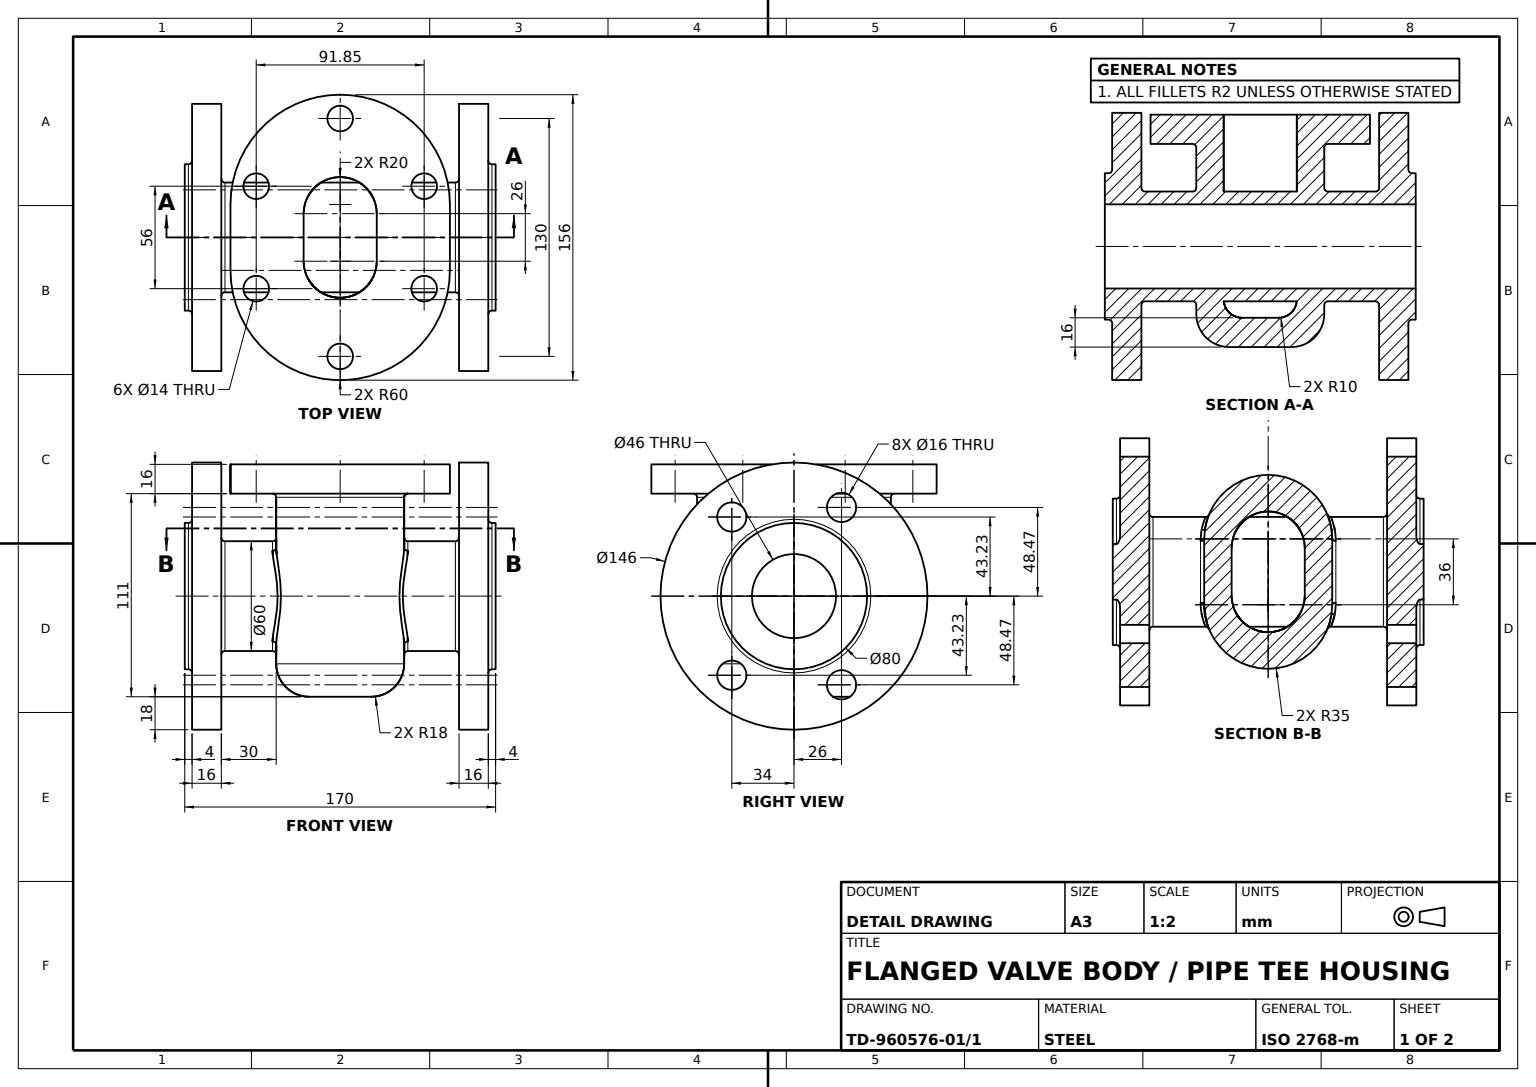
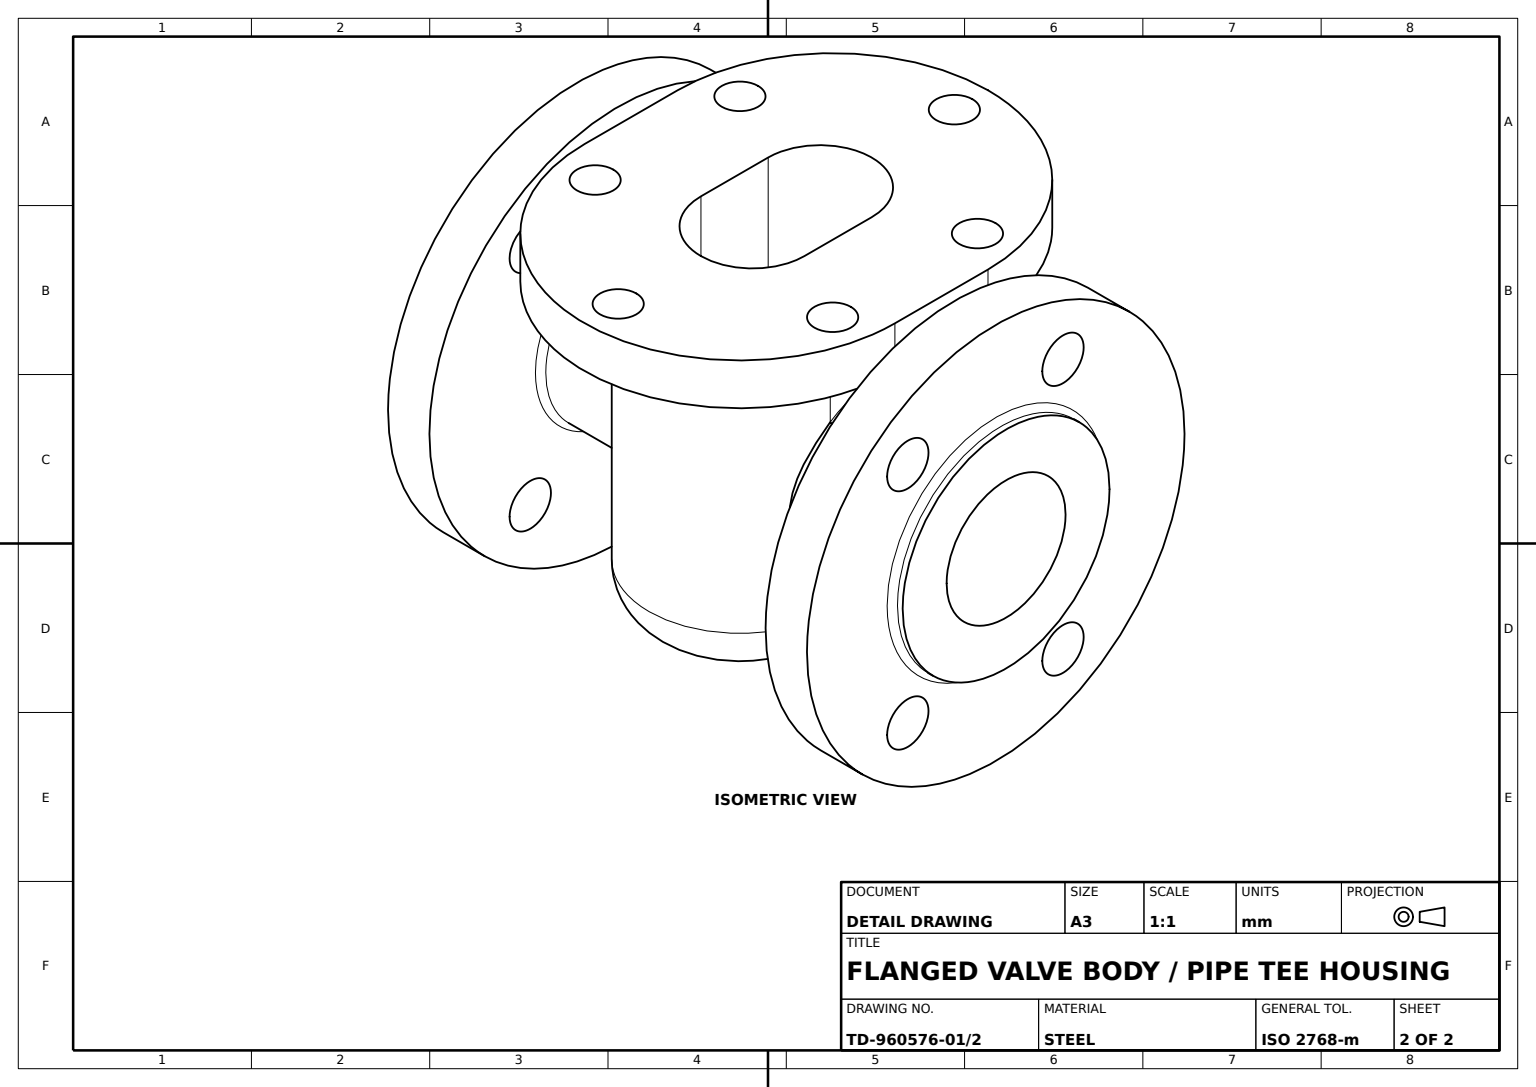
SolidWorks part; units mm, degrees
material "Plain Carbon Steel"
ref_plane "Front Plane" through (0, 0, 0) normal (0, 0, 1) x (1, 0, 0)
ref_plane "Top Plane" through (0, 0, 0) normal (0, 1, 0) x (1, 0, 0)
ref_plane "Right Plane" through (0, 0, 0) normal (1, 0, 0) x (0, 0, -1)
sketch "Bonnet Flange Sketch" plane through (0, 0, 0) normal (0, 1, 0) x (1, 0, 0)
  line L0 (0, -18) -> (0, 18) construction
  line L1 (-60, -18) -> (-60, 18)
  line L2 (60, -18) -> (60, 18)
  line L3 (0, -18) -> (0, 18) construction
  line L6 (-47, -18) -> (-47, 18) construction
  line L7 (47, -18) -> (47, 18) construction
  line L8 (0, -80.3) -> (0, 80.3) construction
  arc A0 (-60, -18) -> (60, -18) centre (0, -18) ccw
  arc A1 (60, 18) -> (-60, 18) centre (0, 18) ccw
  arc A4 (-47, -18) -> (47, -18) centre (0, -18) ccw construction
  arc A5 (47, 18) -> (-47, 18) centre (0, 18) ccw construction
  circle A6 centre (0, 65) radius 7
  circle A7 centre (0, -65) radius 7
  circle A8 centre (45.9239, 28) radius 7
  circle A9 centre (45.9239, -28) radius 7
  circle A10 centre (-45.9239, 28) radius 7
  circle A11 centre (-45.9239, -28) radius 7
  point P2 (0, 0)
  point P10 (0, 0)
  dimension "D1" = 60
  dimension "D2" = 47
  dimension "D4" = 14
  dimension "D3" = 36
  dimension "D5" = 56
  dimension "D6" = 28
extrude "Bonnet Flange" add sketch "Bonnet Flange Sketch" along normal blind 16
sketch "Neck Sketch" plane through (0, 0, 0) normal (0, -1, 0) x (1, 0, 0)
  line L0 (0, -18) -> (0, 18) construction
  line L1 (-35, -18) -> (-35, 18)
  line L2 (35, -18) -> (35, 18)
  arc A0 (-35, -18) -> (35, -18) centre (0, -18) ccw
  arc A1 (35, 18) -> (-35, 18) centre (0, 18) ccw
  point P2 (0, 0)
  dimension "D1" = 35
  dimension "D2" = 36
extrude "Neck" add sketch "Neck Sketch" along normal blind 111 contours A0 L2 A1 L1
sketch "Neck Slot Bore Sketch" plane through (0, 16, 0) normal (0, 1, 0) x (1, 0, 0)
  line L0 (0, -13) -> (0, 13) construction
  line L1 (-20, -13) -> (-20, 13)
  line L2 (20, -13) -> (20, 13)
  arc A0 (-20, -13) -> (20, -13) centre (0, -13) ccw
  arc A1 (20, 13) -> (-20, 13) centre (0, 13) ccw
  point P2 (0, 0)
  dimension "D1" = 20
  dimension "D2" = 26
extrude "Neck Slot Bore" cut sketch "Neck Slot Bore Sketch" against normal blind 111
fillet "Neck Edge Fillet R18" radius 18 4 edges at (-35, -111, 0) (0, -111, 53) (35, -111, 0) (0, -111, -53)
fillet "Slot Bore Fillet R10" radius 10 4 edges at (-20, -95, 0) (0, -95, -33) (20, -95, 0) (0, -95, 33)
ref_plane "End Flange Plane" through (81, 0, 0) normal (1, 0, 0) x (0, 0, -1)
sketch "End Flange Sketch" plane through (81, 0, 0) normal (1, 0, 0) x (0, 0, -1)
  line L0 (78, 16) -> (18, 16) construction
  circle A0 centre (0, -56) radius 73
  dimension "D1" = 146
  dimension "D2" = 72
extrude "End Flange Ø146" add sketch "End Flange Sketch" against normal blind 16 separate body contours A0
mirror "Opposite End Flange Mirror" about plane through (0, 0, 0) normal (1, 0, 0) of bodies 106
sketch "Barrel Sketch" plane through (81, 0, 0) normal (1, 0, 0) x (0, 0, -1)
  circle A0 centre (0, -56) radius 30
  dimension "D1" = 60
extrude "Barrel Ø60" add sketch "Barrel Sketch" against normal blind 148 contours A0
sketch "Raised Face A Sketch" plane through (81, 0, 0) normal (1, 0, 0) x (0, 0, -1)
  circle A0 centre (0, -56) radius 40
  dimension "D1" = 80
extrude "Raised Face A Ø80" add sketch "Raised Face A Sketch" along normal blind 4
sketch "Raised Face B Sketch" plane through (-81, 0, 0) normal (-1, 0, 0) x (0, 0, 1)
  circle A0 centre (0, -56) radius 40
  dimension "D1" = 80
extrude "Raised Face B Ø80" add sketch "Raised Face B Sketch" along normal blind 4
sketch "Through Bore Sketch" plane through (-85, 0, 0) normal (-1, 0, 0) x (0, 0, 1)
  circle A0 centre (0, -56) radius 23
  dimension "D1" = 46
extrude "Through Bore Ø46" cut sketch "Through Bore Sketch" against normal blind 174
fillet "Raised Face Fillets R2" radius 2 2 edges at (81, -56, -40) (-81, -56, 40)
fillet "Barrel Flange Fillets R2" radius 2 2 edges at (65, -56, -30) (-65, -56, 30)
sketch "Flange Bolt Holes Sketch" plane through (81, 0, 0) normal (1, 0, 0) x (0, 0, -1)
  line L0 (0, -56) -> (102.9788, -56) construction
  circle A0 centre (26, -104.4665) radius 8
  circle A1 centre (-34, -99.2319) radius 8
  circle A2 centre (0, -56) radius 55 construction
  circle A3 centre (-34, -12.7681) radius 8
  circle A4 centre (26, -7.5335) radius 8
  dimension "D1" = 110
  dimension "D4" = 16
  dimension "D2" = 60
  dimension "D3" = 26
extrude "Flange Bolt Holes" cut sketch "Flange Bolt Holes Sketch" against normal blind 16 contours A4
mirror "Flange Bolt Holes Mirror" about plane through (0, 0, 0) normal (1, 0, 0) of "Flange Bolt Holes"
fillet "Neck Bonnet Fillet R2" radius 2 4 edges at (-35, 0, 0) (0, 0, 53) (35, 0, 0) (0, 0, -53)
fillet "Neck Barrel Fillet R2" radius 2 8 edges at (35, -26, 0) (35, -86, 0) (32.9259, -53.2049, 29.8695) (-35, -26, 0) (-35, -86, 0) (-32.8894, -54.6657, 29.9703) (32.8894, -54.6657, -29.9703) (-32.9259, -53.2049, -29.8695)
